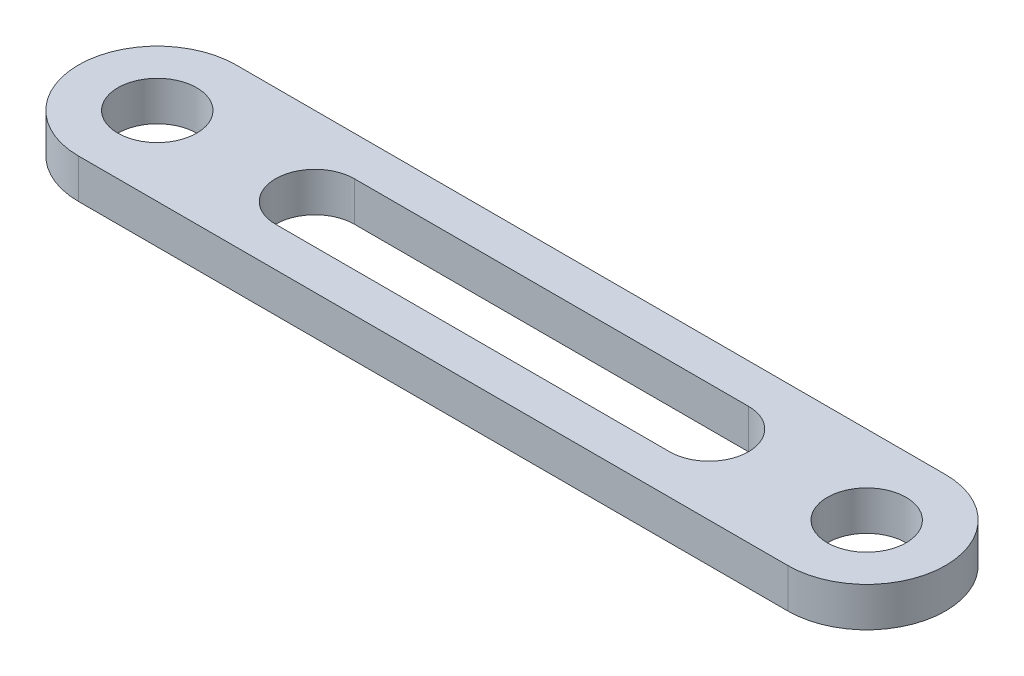
SolidWorks part; units mm, degrees
material "Plain Carbon Steel"
ref_plane "Front Plane" through (0, 0, 0) normal (0, 0, 1) x (1, 0, 0)
ref_plane "Top Plane" through (0, 0, 0) normal (0, 1, 0) x (1, 0, 0)
ref_plane "Right Plane" through (0, 0, 0) normal (1, 0, 0) x (0, 0, -1)
sketch "Link Profile Sketch" plane through (0, 0, 0) normal (0, 1, 0) x (1, 0, 0)
  line L0 (-45, 0) -> (45, 0) construction
  line L1 (-45, 10) -> (45, 10)
  line L2 (-45, -10) -> (45, -10)
  line L3 (-25, 0) -> (25, 0) construction
  line L4 (-25, 5) -> (25, 5)
  line L5 (-25, -5) -> (25, -5)
  arc A0 (-45, 10) -> (-45, -10) centre (-45, 0) ccw
  arc A1 (45, -10) -> (45, 10) centre (45, 0) ccw
  circle A2 centre (-45, 0) radius 5
  circle A3 centre (45, 0) radius 5
  arc A4 (-25, 5) -> (-25, -5) centre (-25, 0) ccw
  arc A5 (25, -5) -> (25, 5) centre (25, 0) ccw
  point P2 (0, 0)
  point P14 (0, 0)
  dimension "D1" = 10
  dimension "D3" = 10
  dimension "D4" = 10
  dimension "D6" = 5
  dimension "D2" = 90
  dimension "D5" = 20
extrude "Link Plate 5mm" add sketch "Link Profile Sketch" along normal blind 5
